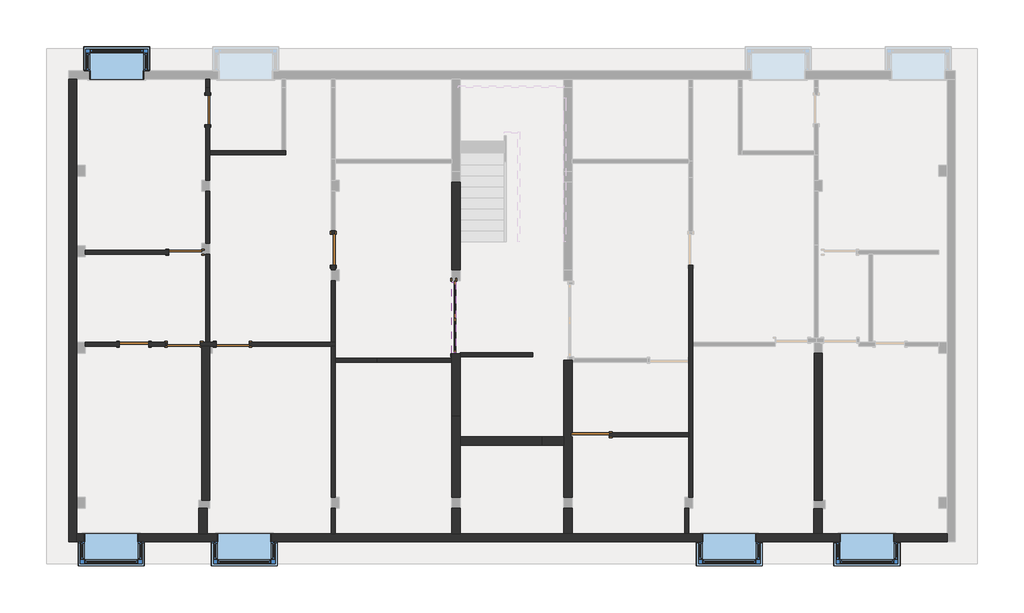
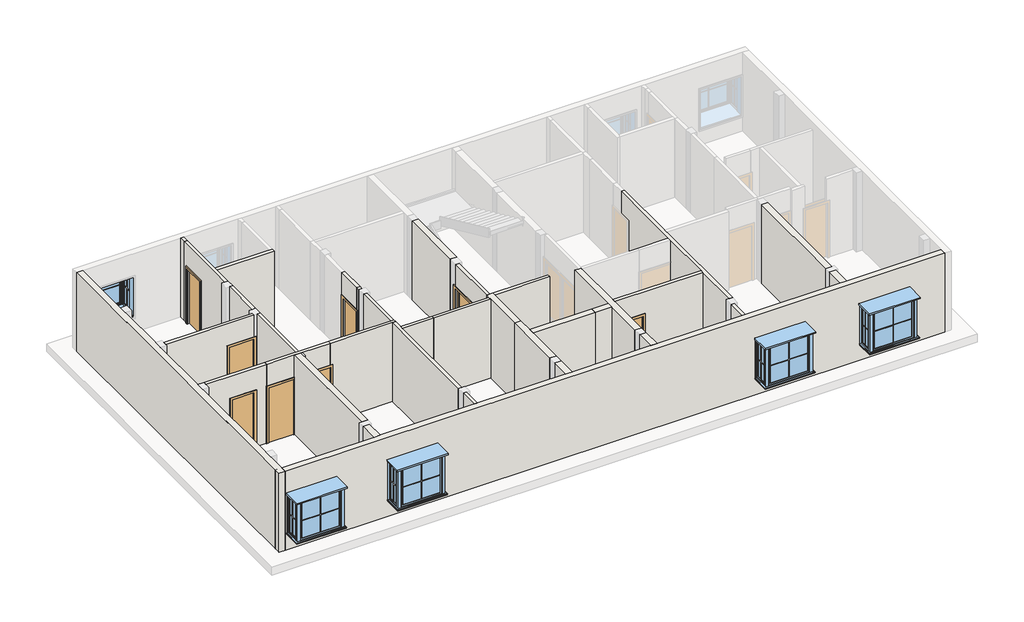
# One storey, part 1 of 3: 36 walls, 8 doors, 5 windows.
"""IFC4 building model written with IfcOpenShell, lengths in millimetres."""

from ifc_helpers import new_model, si_unit, frame, origin, place, context, project, spatial, polyline, outline, extrude, faceted_brep, transform, mapped, element, save
from components import door_b125cbd4, m_door_single_panel_05506f71, door_07b5d71c, door_4c0a2014, door_82def9da, m_door_single_panel_3_x7_f8176753, m_door_single_panel_3_x7_ebb67e73, window_19bbd869

model = new_model("IFC4")

# Units and contexts
model_context = context("Model", 3, world=origin())
ifc_project = project(units=[si_unit("LENGTHUNIT", "METRE", prefix="MILLI")], contexts=[model_context])

# Site, building, storey
site = spatial("IfcSite", under=ifc_project)
building = spatial("IfcBuilding", under=site)
storey = spatial("IfcBuildingStorey", under=building, Elevation=19202.4)

# Doors
placement = place(None, origin())
door_shape = door_b125cbd4(model_context)
element("IfcDoor", 1, ObjectType="M_Door-Double-Glass : 6'7\"X7'", at=placement, inside=storey, context=model_context, shape_type="MappedRepresentation", body=[
    mapped(door_shape, transform((-2022.6300498, 1267.5192699, 19202.4), x_axis=(0.0, 1.0, 0.0), y_axis=(-1.0, 0.0, 0.0), z_axis=(0.0, 0.0, 1.0))),
])
m_door_single_panel_shape = m_door_single_panel_05506f71(model_context)
element("IfcDoor", 2, ObjectType="M_Door-Single-Panel", at=placement, inside=storey, context=model_context, shape_type="MappedRepresentation", body=[
    mapped(m_door_single_panel_shape, transform((1745.3012085, -1975.7432663, 19202.4), x_axis=(-1.0, 0.0, 0.0), y_axis=(0.0, -1.0, 0.0), z_axis=(0.0, 0.0, 1.0))),
])
door_2_shape = door_07b5d71c(model_context)
element("IfcDoor", 3, ObjectType="M_Door-Single-Panel : 2'10\"X7' 2", at=placement, inside=storey, context=model_context, shape_type="MappedRepresentation", body=[
    mapped(door_2_shape, transform((-5360.3487995, 3142.9626891, 19202.4), x_axis=(0.0, -1.0, 0.0), y_axis=(1.0, 0.0, 0.0), z_axis=(0.0, 0.0, 1.0))),
])
door_3_shape = door_4c0a2014(model_context)
element("IfcDoor", 4, ObjectType="M_Door-Single-Panel : 2'8\"X7'", at=placement, inside=storey, context=model_context, shape_type="MappedRepresentation", body=[
    mapped(door_3_shape, transform((-10873.4462614, 526.1567334, 19202.4), x_axis=(1.0, 0.0, 0.0), y_axis=(0.0, 1.0, 0.0), z_axis=(0.0, 0.0, 1.0))),
])
door_4_shape = door_82def9da(model_context)
element("IfcDoor", 5, ObjectType="M_Door-Single-Panel : 2'8\"X7'", at=placement, inside=storey, context=model_context, shape_type="MappedRepresentation", body=[
    mapped(door_4_shape, transform((-8827.4487992, 7008.6751452, 19202.4), x_axis=(0.0, 1.0, 0.0), y_axis=(-1.0, 0.0, 0.0), z_axis=(0.0, 0.0, 1.0))),
])
m_door_single_panel_3_x7_shape = m_door_single_panel_3_x7_f8176753(model_context)
element("IfcDoor", 6, ObjectType="M_Door-Single-Panel : 3'X7'", at=placement, inside=storey, context=model_context, shape_type="MappedRepresentation", body=[
    mapped(m_door_single_panel_3_x7_shape, transform((-9456.0987989, 3078.8567332, 19202.4), x_axis=(1.0, 0.0, 0.0), y_axis=(0.0, 1.0, 0.0), z_axis=(0.0, 0.0, 1.0))),
])
element("IfcDoor", 7, ObjectType="M_Door-Single-Panel : 3'X7'", at=placement, inside=storey, context=model_context, shape_type="MappedRepresentation", body=[
    mapped(m_door_single_panel_3_x7_shape, transform((-8144.8381465, 526.1567334, 19202.4), x_axis=(-1.0, 0.0, 0.0), y_axis=(0.0, -1.0, 0.0), z_axis=(0.0, 0.0, 1.0))),
])
m_door_single_panel_3_x7_2_shape = m_door_single_panel_3_x7_ebb67e73(model_context)
element("IfcDoor", 8, ObjectType="M_Door-Single-Panel : 3'X7'", at=placement, inside=storey, context=model_context, shape_type="MappedRepresentation", body=[
    mapped(m_door_single_panel_3_x7_2_shape, transform((-9494.1987992, 526.1567334, 19202.4), x_axis=(1.0, 0.0, 0.0), y_axis=(0.0, 1.0, 0.0), z_axis=(0.0, 0.0, 1.0))),
])

# Walls
element("IfcWall", 9, ObjectType="4.5\"", at=placement, inside=storey, context=model_context, shape_type="SweptSolid", body=[
    extrude(outline(polyline([(2711.1626891, 22250.4), (3671.8272228, 22250.4), (3671.8272228, 19202.4), (3574.7626891, 19202.4), (3574.7626891, 21336.0), (2711.1626891, 21336.0), (2711.1626891, 22250.4)])), frame((-5417.4987995, 0.0, 0.0), z_axis=(1.0, 0.0, 0.0), x_axis=(0.0, 1.0, 0.0)), (0.0, 0.0, 1.0), 114.3),
])
element("IfcWall", 10, ObjectType="4.5\"", at=placement, inside=storey, context=model_context, shape_type="Brep", body=[
    faceted_brep([(-7690.1644155, 469.0067334, 22250.4), (-8713.148796, 469.0067334, 22250.4), (-8771.750543, 469.0067334, 22250.4), (-9000.350543, 469.0067334, 22250.4), (-10009.8462614, 469.0067334, 22250.4), (-10009.8462614, 469.0067334, 19202.4), (-9951.3987992, 469.0067334, 19202.4), (-9951.3987992, 469.0067334, 21336.0), (-9036.9987992, 469.0067334, 21336.0), (-9036.9987992, 469.0067334, 19202.4), (-9000.350543, 469.0067334, 19202.4), (-8771.750543, 469.0067334, 19202.4), (-8713.148796, 469.0067334, 19202.4), (-8602.0381465, 469.0067334, 19202.4), (-8602.0381465, 469.0067334, 21336.0), (-7690.1644155, 469.0067334, 21336.0), (-10009.8462614, 583.3067334, 22250.4), (-7690.1644155, 583.3067334, 22250.4), (-7690.1644155, 583.3067334, 21336.0), (-8602.0381465, 583.3067334, 21336.0), (-8602.0381465, 583.3067334, 19202.4), (-9036.9987992, 583.3067334, 19202.4), (-9036.9987992, 583.3067334, 21336.0), (-9951.3987992, 583.3067334, 21336.0), (-9951.3987992, 583.3067334, 19202.4), (-10009.8462614, 583.3067334, 19202.4)], [[[0, 1, 2, 3, 4, 5, 6, 7, 8, 9, 10, 11, 12, 13, 14, 15]], [[16, 17, 18, 19, 20, 21, 22, 23, 24, 25]], [[5, 25, 24, 6]], [[9, 21, 20, 13, 12, 11, 10]], [[17, 0, 15, 18]], [[4, 3, 2, 1, 0, 17, 16]], [[5, 4, 16, 25]], [[8, 22, 21, 9]], [[7, 23, 22, 8]], [[23, 7, 6, 24]], [[19, 14, 13, 20]], [[14, 19, 18, 15]]]),
])
element("IfcWall", 11, ObjectType="4.5\"", at=placement, inside=storey, context=model_context, shape_type="SweptSolid", body=[
    extrude(outline(polyline([(22250.4, 4475.8012082), (22250.4, 1250.0012085), (21336.0, 1250.0012085), (21336.0, 2278.7012085), (19202.4, 2278.7012085), (19202.4, 4475.8012082), (22250.4, 4475.8012082)])), frame((0.0, -2032.8932663, 0.0), z_axis=(0.0, 1.0, 0.0), x_axis=(0.0, 0.0, 1.0)), (0.0, 0.0, 1.0), 114.3),
])
element("IfcWall", 12, ObjectType="4.5\"", at=placement, inside=storey, context=model_context, shape_type="Brep", body=[
    faceted_brep([(-5417.4987995, 469.0067334, 19202.4), (-5417.4987995, -3709.2932193, 19202.4), (-5417.4987995, -3709.2932193, 22250.4), (-5417.4987995, 469.0067334, 22250.4), (-5303.1987995, 469.0067334, 19202.4), (-5303.1987995, 469.0067334, 22250.4), (-5303.1987995, 148.1078621, 22250.4), (-5303.1987995, 33.8078621, 22250.4), (-5303.1987995, -3709.2932193, 22250.4), (-5303.1987995, -3709.2932193, 19202.4), (-5303.1987995, 33.8078621, 19202.4), (-5303.1987995, 148.1078621, 19202.4)], [[[0, 1, 2, 3]], [[4, 5, 6, 7, 8, 9, 10, 11]], [[1, 0, 4, 11, 10, 9]], [[2, 1, 9, 8]], [[3, 2, 8, 7, 6, 5]], [[0, 3, 5, 4]]]),
])
element("IfcWall", 13, ObjectType="4.5\"", at=placement, inside=storey, context=model_context, shape_type="SweptSolid", body=[
    extrude(outline(polyline([(-5417.4987963, -4712.5932661), (-5417.4987963, -4014.0932193), (-5303.1987963, -4014.0932193), (-5303.1987963, -4712.5932661), (-5417.4987963, -4712.5932661)])), frame((0.0, 0.0, 19202.4), z_axis=(0.0, 0.0, 1.0), x_axis=(1.0, 0.0, 0.0)), (0.0, 0.0, 1.0), 3048.0),
])
element("IfcWall", 14, ObjectType="4.5\"", at=placement, inside=storey, context=model_context, shape_type="SweptSolid", body=[
    extrude(outline(polyline([(4361.5012082, -4712.5932661), (4361.5012082, -4014.0932193), (4475.8012082, -4014.0932193), (4475.8012082, -4712.5932661), (4361.5012082, -4712.5932661)])), frame((0.0, 0.0, 19202.4), z_axis=(0.0, 0.0, 1.0), x_axis=(1.0, 0.0, 0.0)), (0.0, 0.0, 1.0), 3048.0),
])
element("IfcWall", 15, ObjectType="4.5\"", at=placement, inside=storey, context=model_context, shape_type="SweptSolid", body=[
    extrude(outline(polyline([(-8770.2987992, 7860.4067329), (-8770.2987992, 7631.8067329), (-8884.5987992, 7631.8067329), (-8884.5987992, 7860.4067329), (-8770.2987992, 7860.4067329)])), frame((0.0, 0.0, 19202.4), z_axis=(0.0, 0.0, 1.0), x_axis=(1.0, 0.0, 0.0)), (0.0, 0.0, 1.0), 3048.0),
])
element("IfcWall", 16, ObjectType="4.5\"", at=placement, inside=storey, context=model_context, shape_type="SweptSolid", body=[
    extrude(outline(polyline([(-5303.1987995, 148.1078621), (-4161.4090098, 148.1078621), (-4161.4090098, 33.8078621), (-5303.1987995, 33.8078621), (-5303.1987995, 148.1078621)])), frame((0.0, 0.0, 19202.4), z_axis=(0.0, 0.0, 1.0), x_axis=(1.0, 0.0, 0.0)), (0.0, 0.0, 1.0), 3048.0),
])
element("IfcWall", 17, ObjectType="4.5\"", at=placement, inside=storey, context=model_context, shape_type="Brep", body=[
    faceted_brep([(154.7082462, 294.3817656, 19202.4), (-1848.7987998, 294.3817656, 19202.4), (-1848.7987998, 294.3817656, 21336.0), (-1848.7987998, 294.3817656, 22250.4), (154.7082462, 294.3817656, 22250.4), (154.7082462, 180.0817656, 19202.4), (154.7082462, 180.0817656, 22250.4), (-1848.7987998, 180.0817656, 22250.4), (-1848.7987998, 180.0817656, 19202.4), (-1848.7987998, 264.2192699, 19202.4)], [[[0, 1, 2, 3, 4]], [[5, 6, 7, 8]], [[1, 0, 5, 8, 9]], [[4, 3, 7, 6]], [[0, 4, 6, 5]], [[3, 2, 1, 9, 8, 7]]]),
])
element("IfcWall", 18, ObjectType="4.5\"", at=placement, inside=storey, context=model_context, shape_type="SweptSolid", body=[
    extrude(outline(polyline([(-1963.0987998, 2240.6567742), (-1963.0987998, 294.3817656), (-2077.3987998, 294.3817656), (-2077.3987998, 2240.6567742), (-1963.0987998, 2240.6567742)])), frame((0.0, 0.0, 21336.0), z_axis=(0.0, 0.0, 1.0), x_axis=(1.0, 0.0, 0.0)), (0.0, 0.0, 1.0), 914.4),
])
element("IfcWall", 19, ObjectType="4.5\" 2", at=placement, inside=storey, context=model_context, shape_type="SweptSolid", body=[
    extrude(outline(polyline([(22250.4, -8998.8987989), (22250.4, -12224.6987989), (19202.4, -12224.6987989), (19202.4, -9913.2987989), (21336.0, -9913.2987989), (21336.0, -8998.8987989), (22250.4, -8998.8987989)])), frame((0.0, 3021.7067332, 0.0), z_axis=(0.0, 1.0, 0.0), x_axis=(0.0, 0.0, 1.0)), (0.0, 0.0, 1.0), 114.3),
])
element("IfcWall", 20, ObjectType="4.5\" 2", at=placement, inside=storey, context=model_context, shape_type="SweptSolid", body=[
    extrude(outline(polyline([(-8770.2987992, 4761.606733), (-8770.2987992, 3326.5067332), (-8884.5987992, 3326.5067332), (-8884.5987992, 4761.606733), (-8770.2987992, 4761.606733)])), frame((0.0, 0.0, 19202.4), z_axis=(0.0, 0.0, 1.0), x_axis=(1.0, 0.0, 0.0)), (0.0, 0.0, 1.0), 3048.0),
])
element("IfcWall", 21, ObjectType="4.5\" 2", at=placement, inside=storey, context=model_context, shape_type="Brep", body=[
    faceted_brep([(-8770.2987992, 7415.0751452, 21336.0), (-8770.2987992, 7415.0751452, 19202.4), (-8770.2987992, 7631.8067329, 19202.4), (-8770.2987992, 7631.8067329, 22250.4), (-8770.2987992, 5879.2067329, 22250.4), (-8770.2987992, 5764.9067329, 22250.4), (-8770.2987992, 5066.406733, 22250.4), (-8770.2987992, 5066.406733, 19202.4), (-8770.2987992, 5764.9067329, 19202.4), (-8770.2987992, 5879.2067329, 19202.4), (-8770.2987992, 6602.2751452, 19202.4), (-8770.2987992, 6602.2751452, 21336.0), (-8884.5987992, 7631.8067329, 19202.4), (-8884.5987992, 7415.0751452, 19202.4), (-8884.5987992, 7415.0751452, 21336.0), (-8884.5987992, 6602.2751452, 21336.0), (-8884.5987992, 6602.2751452, 19202.4), (-8884.5987992, 5066.406733, 19202.4), (-8884.5987992, 5066.406733, 22250.4), (-8884.5987992, 7631.8067329, 22250.4)], [[[0, 1, 2, 3, 4, 5, 6, 7, 8, 9, 10, 11]], [[12, 13, 14, 15, 16, 17, 18, 19]], [[2, 1, 13, 12]], [[10, 9, 8, 7, 17, 16]], [[3, 2, 12, 19]], [[6, 5, 4, 3, 19, 18]], [[7, 6, 18, 17]], [[14, 13, 1, 0]], [[15, 14, 0, 11]], [[16, 15, 11, 10]]]),
])
element("IfcWall", 22, ObjectType="4.5\" 2", at=placement, inside=storey, context=model_context, shape_type="Brep", body=[
    faceted_brep([(-8770.2987992, 5764.9067329, 19202.4), (-6674.7987994, 5764.9067329, 19202.4), (-6674.7987994, 5764.9067329, 22250.4), (-8770.2987992, 5764.9067329, 22250.4), (-8770.2987992, 5879.2067329, 19202.4), (-8770.2987992, 5879.2067329, 22250.4), (-6789.0987994, 5879.2067329, 22250.4), (-6674.7987994, 5879.2067329, 22250.4), (-6674.7987994, 5879.2067329, 19202.4), (-6789.0987994, 5879.2067329, 19202.4)], [[[0, 1, 2, 3]], [[4, 5, 6, 7, 8, 9]], [[1, 0, 4, 9, 8]], [[3, 2, 7, 6, 5]], [[0, 3, 5, 4]], [[2, 1, 8, 7]]]),
])
element("IfcWall", 23, ObjectType="4.5\" 2", at=placement, inside=storey, context=model_context, shape_type="SweptSolid", body=[
    extrude(outline(polyline([(21336.0, -10467.0462614), (19202.4, -10467.0462614), (19202.4, -10009.8462614), (22250.4, -10009.8462614), (22250.4, -12224.6987989), (19202.4, -12224.6987989), (19202.4, -11279.8462614), (21336.0, -11279.8462614), (21336.0, -10467.0462614)])), frame((0.0, 469.0067334, 0.0), z_axis=(0.0, 1.0, 0.0), x_axis=(0.0, 0.0, 1.0)), (0.0, 0.0, 1.0), 114.3),
])
element("IfcWall", 24, ObjectType="4.5\" 2", at=placement, inside=storey, context=model_context, shape_type="SweptSolid", body=[
    extrude(outline(polyline([(-8770.298796, 3021.7067332), (-8770.298796, 583.3067804), (-8884.598796, 583.3067804), (-8884.598796, 3021.7067332), (-8770.298796, 3021.7067332)])), frame((0.0, 0.0, 19202.4), z_axis=(0.0, 0.0, 1.0), x_axis=(1.0, 0.0, 0.0)), (0.0, 0.0, 1.0), 3048.0),
])
element("IfcWall", 25, ObjectType="4.5\" 2", at=placement, inside=storey, context=model_context, shape_type="Brep", body=[
    faceted_brep([(-5303.1987995, 469.0067334, 22250.4), (-5417.4987995, 469.0067334, 22250.4), (-7690.1644155, 469.0067334, 22250.4), (-7690.1644155, 469.0067334, 21336.0), (-7687.6381465, 469.0067334, 21336.0), (-7687.6381465, 469.0067334, 19202.4), (-5417.4987995, 469.0067334, 19202.4), (-5303.1987995, 469.0067334, 19202.4), (-7690.1644155, 583.3067334, 22250.4), (-5417.4987995, 583.3067334, 22250.4), (-5303.1987995, 583.3067334, 22250.4), (-5303.1987995, 583.3067334, 19202.4), (-5417.4987995, 583.3067334, 19202.4), (-7687.6381465, 583.3067334, 19202.4), (-7687.6381465, 583.3067334, 21336.0), (-7690.1644155, 583.3067334, 21336.0)], [[[0, 1, 2, 3, 4, 5, 6, 7]], [[8, 9, 10, 11, 12, 13, 14, 15]], [[11, 7, 6, 5, 13, 12]], [[2, 1, 0, 10, 9, 8]], [[2, 8, 15, 3]], [[0, 7, 11, 10]], [[14, 4, 3, 15]], [[4, 14, 13, 5]]]),
])
element("IfcWall", 26, ObjectType="4.5\" 2", at=placement, inside=storey, context=model_context, shape_type="SweptSolid", body=[
    extrude(outline(polyline([(-5303.1987995, 2285.1067802), (-5303.1987995, 583.3067334), (-5417.4987995, 583.3067334), (-5417.4987995, 2285.1067802), (-5303.1987995, 2285.1067802)])), frame((0.0, 0.0, 19202.4), z_axis=(0.0, 0.0, 1.0), x_axis=(1.0, 0.0, 0.0)), (0.0, 0.0, 1.0), 3048.0),
])
element("IfcWall", 27, ObjectType="4.5\" 2", at=placement, inside=storey, context=model_context, shape_type="Brep", body=[
    faceted_brep([(-5303.1987995, 2589.9067802, 19202.4), (-5303.1987995, 2711.1626891, 19202.4), (-5303.1987995, 2711.1626891, 21336.0), (-5303.1987995, 2711.1626891, 22250.4), (-5303.1987995, 2589.9067802, 22250.4), (-5417.4987995, 2589.9067802, 19202.4), (-5417.4987995, 2589.9067802, 22250.4), (-5417.4987995, 2711.1626891, 22250.4), (-5417.4987995, 2711.1626891, 21336.0), (-5417.4987995, 2711.1626891, 19202.4)], [[[0, 1, 2, 3, 4]], [[5, 6, 7, 8, 9]], [[1, 0, 5, 9]], [[3, 2, 1, 9, 8, 7]], [[4, 3, 7, 6]], [[0, 4, 6, 5]]]),
])
element("IfcWall", 28, ObjectType="4.5\" 2", at=placement, inside=storey, context=model_context, shape_type="Brep", body=[
    faceted_brep([(4475.8012082, -3709.2932193, 19202.4), (4475.8012082, -3709.2932193, 22250.4), (4475.8012082, -2032.8932663, 22250.4), (4475.8012082, -1918.5932663, 22250.4), (4475.8012082, 33.8078621, 22250.4), (4475.8012082, 148.1078621, 22250.4), (4475.8012082, 3132.0737955, 22250.4), (4475.8012082, 3132.0737955, 21336.0), (4475.8012082, 2711.1626891, 21336.0), (4475.8012082, 2711.1626891, 19202.4), (4475.8012082, 148.1078621, 19202.4), (4475.8012082, 33.8078621, 19202.4), (4475.8012082, -1918.5932663, 19202.4), (4475.8012082, -2032.8932663, 19202.4), (4590.1012082, -3709.2932193, 22250.4), (4590.1012082, -3709.2932193, 19202.4), (4590.1012082, 469.0067334, 19202.4), (4590.1012082, 583.3067334, 19202.4), (4590.1012082, 2711.1626891, 19202.4), (4590.1012082, 2711.1626891, 21336.0), (4590.1012082, 3132.0737955, 21336.0), (4590.1012082, 3132.0737955, 22250.4), (4590.1012082, 583.3067334, 22250.4), (4590.1012082, 469.0067334, 22250.4)], [[[0, 1, 2, 3, 4, 5, 6, 7, 8, 9, 10, 11, 12, 13]], [[14, 15, 16, 17, 18, 19, 20, 21, 22, 23]], [[15, 0, 13, 12, 11, 10, 9, 18, 17, 16]], [[1, 0, 15, 14]], [[6, 5, 4, 3, 2, 1, 14, 23, 22, 21]], [[6, 21, 20, 7]], [[8, 19, 18, 9]], [[19, 8, 7, 20]]]),
])
element("IfcWall", 29, ObjectType="4.5\" 2", at=placement, inside=storey, context=model_context, shape_type="SweptSolid", body=[
    extrude(outline(polyline([(-2077.3987998, 33.8078621), (-4161.4090098, 33.8078621), (-4161.4090098, 148.1078621), (-2077.3987998, 148.1078621), (-2077.3987998, 33.8078621)])), frame((0.0, 0.0, 19202.4), z_axis=(0.0, 0.0, 1.0), x_axis=(1.0, 0.0, 0.0)), (0.0, 0.0, 1.0), 3048.0),
])
element("IfcWall", 30, ObjectType="9\"", at=placement, inside=storey, context=model_context, shape_type="Brep", body=[
    faceted_brep([(-12453.2987957, -4941.1932661, 19202.4), (-12453.2987957, -4712.5932661, 19202.4), (-12453.2987957, -4014.0932671, 19202.4), (-12453.2987957, -3709.2932671, 19202.4), (-12453.2987957, 278.5067334, 19202.4), (-12453.2987957, 583.3067334, 19202.4), (-12453.2987957, 2951.8567332, 19202.4), (-12453.2987957, 3256.6567332, 19202.4), (-12453.2987957, 5174.3567339, 19202.4), (-12453.2987957, 5479.1567339, 19202.4), (-12453.2987957, 7860.4067329, 19202.4), (-12453.2987957, 7860.4067329, 22250.4), (-12453.2987957, 5479.1567339, 22250.4), (-12453.2987957, 5174.3567339, 22250.4), (-12453.2987957, 3256.6567332, 22250.4), (-12453.2987957, 2951.8567332, 22250.4), (-12453.2987957, 583.3067334, 22250.4), (-12453.2987957, 278.5067334, 22250.4), (-12453.2987957, -3709.2932671, 22250.4), (-12453.2987957, -4014.0932671, 22250.4), (-12453.2987957, -4712.5932661, 22250.4), (-12453.2987957, -4941.1932661, 22250.4), (-12681.8987957, -4941.1932661, 19202.4), (-12681.8987957, -4941.1932661, 22250.4), (-12681.8987957, 7860.4067329, 22250.4), (-12681.8987957, 7860.4067329, 19202.4)], [[[0, 1, 2, 3, 4, 5, 6, 7, 8, 9, 10, 11, 12, 13, 14, 15, 16, 17, 18, 19, 20, 21]], [[22, 23, 24, 25]], [[10, 9, 8, 7, 6, 5, 4, 3, 2, 1, 0, 22, 25]], [[21, 20, 19, 18, 17, 16, 15, 14, 13, 12, 11, 24, 23]], [[11, 10, 25, 24]], [[0, 21, 23, 22]]]),
])
element("IfcWall", 31, ObjectType="9\"", at=placement, inside=storey, context=model_context, shape_type="Brep", body=[
    faceted_brep([(-12453.2987957, -4712.5932661, 19202.4), (-12453.2987957, -4014.0932671, 19202.4), (-12453.2987957, -3709.2932671, 19202.4), (-12453.2987957, 278.5067334, 19202.4), (-12453.2987957, 583.3067334, 19202.4), (-12453.2987957, 2951.8567332, 19202.4), (-12453.2987957, 3256.6567332, 19202.4), (-12453.2987957, 5174.3567339, 19202.4), (-12453.2987957, 5479.1567339, 19202.4), (-12453.2987957, 7860.4067329, 19202.4), (-12453.2987957, 7860.4067329, 22250.4), (-12453.2987957, 5479.1567339, 22250.4), (-12453.2987957, 5174.3567339, 22250.4), (-12453.2987957, 3256.6567332, 22250.4), (-12453.2987957, 2951.8567332, 22250.4), (-12453.2987957, 583.3067334, 22250.4), (-12453.2987957, 278.5067334, 22250.4), (-12453.2987957, -3709.2932671, 22250.4), (-12453.2987957, -4014.0932671, 22250.4), (-12453.2987957, -4712.5932661, 22250.4), (-12681.8987957, -4712.5932661, 19202.4), (-12681.8987957, -4712.5932661, 22250.4), (-12681.8987957, 7860.4067329, 22250.4), (-12681.8987957, 7860.4067329, 19202.4)], [[[0, 1, 2, 3, 4, 5, 6, 7, 8, 9, 10, 11, 12, 13, 14, 15, 16, 17, 18, 19]], [[20, 21, 22, 23]], [[9, 8, 7, 6, 5, 4, 3, 2, 1, 0, 20, 23]], [[19, 18, 17, 16, 15, 14, 13, 12, 11, 10, 22, 21]], [[10, 9, 23, 22]], [[0, 19, 21, 20]]]),
])
element("IfcWall", 32, ObjectType="9\"", at=placement, inside=storey, context=model_context, shape_type="Brep", body=[
    faceted_brep([(-9000.350543, 469.0067334, 19202.4), (-9000.350543, -3785.4932196, 19202.4), (-9000.350543, -3785.4932196, 22250.4), (-9000.350543, 469.0067334, 22250.4), (-8771.750543, 469.0067334, 19202.4), (-8771.750543, 469.0067334, 22250.4), (-8771.750543, 278.5067334, 22250.4), (-8771.750543, -3785.4932196, 22250.4), (-8771.750543, -3785.4932196, 19202.4), (-8771.750543, 278.5067334, 19202.4)], [[[0, 1, 2, 3]], [[4, 5, 6, 7, 8, 9]], [[1, 0, 4, 9, 8]], [[2, 1, 8, 7]], [[3, 2, 7, 6, 5]], [[0, 3, 5, 4]]]),
])
element("IfcWall", 33, ObjectType="9\"", at=placement, inside=storey, context=model_context, shape_type="Brep", body=[
    faceted_brep([(-2077.3987998, -1469.0258023, 19202.4), (-2077.3987998, -1469.0258023, 22250.4), (-2077.3987998, 33.8078621, 22250.4), (-2077.3987998, 148.1078621, 22250.4), (-2077.3987998, 294.3817656, 22250.4), (-2077.3987998, 294.3817656, 21336.0), (-2077.3987998, 264.2192699, 21336.0), (-2077.3987998, 264.2192699, 19202.4), (-2077.3987998, 148.1078621, 19202.4), (-2077.3987998, 33.8078621, 19202.4), (-1848.7987998, -1469.0258023, 22250.4), (-1848.7987998, -1469.0258023, 19202.4), (-1848.7987998, 180.0817656, 19202.4), (-1848.7987998, 264.2192699, 19202.4), (-1848.7987998, 264.2192699, 21336.0), (-1848.7987998, 294.3817656, 21336.0), (-1848.7987998, 294.3817656, 22250.4), (-1848.7987998, 180.0817656, 22250.4), (-1963.0987998, 294.3817656, 22250.4), (-1963.0987998, 294.3817656, 21336.0)], [[[0, 1, 2, 3, 4, 5, 6, 7, 8, 9]], [[10, 11, 12, 13, 14, 15, 16, 17]], [[11, 0, 9, 8, 7, 13, 12]], [[1, 0, 11, 10]], [[4, 3, 2, 1, 10, 17, 16, 18]], [[4, 18, 16, 15, 19, 5]], [[14, 6, 5, 19, 15]], [[6, 14, 13, 7]]]),
])
element("IfcWall", 34, ObjectType="9\"", at=placement, inside=storey, context=model_context, shape_type="Brep", body=[
    faceted_brep([(-2077.3987998, -1469.0258023, 19202.4), (-2077.3987998, -3709.2932663, 19202.4), (-2077.3987998, -3709.2932663, 22250.4), (-2077.3987998, -1469.0258023, 22250.4), (-1848.7987998, -1469.0258023, 19202.4), (-1848.7987998, -1469.0258023, 22250.4), (-1848.7987998, -2032.8932663, 22250.4), (-1848.7987998, -2261.4932663, 22250.4), (-1848.7987998, -3709.2932663, 22250.4), (-1848.7987998, -3709.2932663, 19202.4), (-1848.7987998, -2261.4932663, 19202.4), (-1848.7987998, -2032.8932663, 19202.4)], [[[0, 1, 2, 3]], [[4, 5, 6, 7, 8, 9, 10, 11]], [[1, 0, 4, 11, 10, 9]], [[2, 1, 9, 8]], [[3, 2, 8, 7, 6, 5]], [[0, 3, 5, 4]]]),
])
element("IfcWall", 35, ObjectType="9\"", at=placement, inside=storey, context=model_context, shape_type="SweptSolid", body=[
    extrude(outline(polyline([(1021.4012085, -2261.4932663), (412.152227, -2261.4932663), (412.152227, -2032.8932663), (1021.4012085, -2032.8932663), (1021.4012085, -2261.4932663)])), frame((0.0, 0.0, 19202.4), z_axis=(0.0, 0.0, 1.0), x_axis=(1.0, 0.0, 0.0)), (0.0, 0.0, 1.0), 3048.0),
])
element("IfcWall", 36, ObjectType="9\"", at=placement, inside=storey, context=model_context, shape_type="Brep", body=[
    faceted_brep([(1021.4012085, 90.9578621, 19202.4), (1021.4012085, -2032.8932663, 19202.4), (1021.4012085, -2261.4932663, 19202.4), (1021.4012085, -3709.2932193, 19202.4), (1021.4012085, -3709.2932193, 22250.4), (1021.4012085, -2261.4932663, 22250.4), (1021.4012085, -2032.8932663, 22250.4), (1021.4012085, 90.9578621, 22250.4), (1250.0012085, -3709.2932193, 22250.4), (1250.0012085, -3709.2932193, 19202.4), (1250.0012085, -2032.8932663, 19202.4), (1250.0012085, -2032.8932663, 21336.0), (1250.0012085, -1918.5932663, 21336.0), (1250.0012085, -1918.5932663, 19202.4), (1250.0012085, 33.8078621, 19202.4), (1250.0012085, 90.9578621, 19202.4), (1250.0012085, 90.9578621, 22250.4), (1250.0012085, 33.8078621, 22250.4), (1250.0012085, -1918.5932663, 22250.4), (1250.0012085, -2032.8932663, 22250.4), (1158.0082462, 90.9578621, 19202.4), (1211.9012085, -1918.5932663, 19202.4), (1211.9012085, -2032.8932663, 19202.4), (1158.0082462, 90.9578621, 22250.4), (1211.9012085, -1918.5932663, 21336.0), (1211.9012085, -2032.8932663, 21336.0)], [[[0, 1, 2, 3, 4, 5, 6, 7]], [[8, 9, 10, 11, 12, 13, 14, 15, 16, 17, 18, 19]], [[3, 2, 1, 0, 20, 15, 14, 13, 21, 22, 10, 9]], [[4, 3, 9, 8]], [[7, 6, 5, 4, 8, 19, 18, 17, 16, 23]], [[0, 7, 23, 16, 15, 20]], [[24, 21, 13, 12]], [[22, 25, 11, 10]], [[21, 24, 25, 22]], [[25, 24, 12, 11]]]),
])
element("IfcWall", 37, ObjectType="9\"", at=placement, inside=storey, context=model_context, shape_type="SweptSolid", body=[
    extrude(outline(polyline([(-2074.1417538, 2589.906774), (-2074.1417538, 5015.606774), (-1845.5417538, 5015.606774), (-1845.5417538, 2589.906774), (-2074.1417538, 2589.906774)])), frame((0.0, 0.0, 19202.4), z_axis=(0.0, 0.0, 1.0), x_axis=(1.0, 0.0, 0.0)), (0.0, 0.0, 1.0), 3048.0),
])
element("IfcWall", 38, ObjectType="9\"", at=placement, inside=storey, context=model_context, shape_type="SweptSolid", body=[
    extrude(outline(polyline([(7942.9012047, -3785.4932666), (7942.9012047, 278.5067334), (8171.5012047, 278.5067334), (8171.5012047, -3785.4932666), (7942.9012047, -3785.4932666)])), frame((0.0, 0.0, 19202.4), z_axis=(0.0, 0.0, 1.0), x_axis=(1.0, 0.0, 0.0)), (0.0, 0.0, 1.0), 3048.0),
])
element("IfcWall", 39, ObjectType="9\"", at=placement, inside=storey, context=model_context, shape_type="SweptSolid", body=[
    extrude(outline(polyline([(1021.4012085, -4712.5932661), (1021.4012085, -4014.0932193), (1250.0012085, -4014.0932193), (1250.0012085, -4712.5932661), (1021.4012085, -4712.5932661)])), frame((0.0, 0.0, 19202.4), z_axis=(0.0, 0.0, 1.0), x_axis=(1.0, 0.0, 0.0)), (0.0, 0.0, 1.0), 3048.0),
])
element("IfcWall", 40, ObjectType="9\"", at=placement, inside=storey, context=model_context, shape_type="SweptSolid", body=[
    extrude(outline(polyline([(7941.7646942, -4712.5932661), (7941.7646942, -4015.9914801), (8170.3646942, -4015.9914801), (8170.3646942, -4712.5932661), (7941.7646942, -4712.5932661)])), frame((0.0, 0.0, 19202.4), z_axis=(0.0, 0.0, 1.0), x_axis=(1.0, 0.0, 0.0)), (0.0, 0.0, 1.0), 3048.0),
])
element("IfcWall", 41, ObjectType="9\"", at=placement, inside=storey, context=model_context, shape_type="SweptSolid", body=[
    extrude(outline(polyline([(-2077.3987998, -4712.5932661), (-2077.3987998, -4014.0932663), (-1848.7987998, -4014.0932663), (-1848.7987998, -4712.5932661), (-2077.3987998, -4712.5932661)])), frame((0.0, 0.0, 19202.4), z_axis=(0.0, 0.0, 1.0), x_axis=(1.0, 0.0, 0.0)), (0.0, 0.0, 1.0), 3048.0),
])
element("IfcWall", 42, ObjectType="9\"", at=placement, inside=storey, context=model_context, shape_type="SweptSolid", body=[
    extrude(outline(polyline([(-9076.550543, -4712.5932661), (-9076.550543, -4014.0932196), (-8847.950543, -4014.0932196), (-8847.950543, -4712.5932661), (-9076.550543, -4712.5932661)])), frame((0.0, 0.0, 19202.4), z_axis=(0.0, 0.0, 1.0), x_axis=(1.0, 0.0, 0.0)), (0.0, 0.0, 1.0), 3048.0),
])
element("IfcWall", 43, ObjectType="9\"", at=placement, inside=storey, context=model_context, shape_type="SweptSolid", body=[
    extrude(outline(polyline([(-1848.7987998, -2032.8932663), (412.152227, -2032.8932663), (412.152227, -2261.4932663), (-1848.7987998, -2261.4932663), (-1848.7987998, -2032.8932663)])), frame((0.0, 0.0, 19202.4), z_axis=(0.0, 0.0, 1.0), x_axis=(1.0, 0.0, 0.0)), (0.0, 0.0, 1.0), 3048.0),
])
element("IfcWall", 44, ObjectType="9\" 2", at=placement, inside=storey, context=model_context, shape_type="Brep", body=[
    faceted_brep([(-12453.2987957, -4941.1932661, 19202.4), (11625.9012075, -4941.1932662, 19202.4), (11625.9012075, -4941.1932662, 22250.4), (-12453.2987957, -4941.1932661, 22250.4), (8658.6146942, -4941.1932661, 21353.2), (10158.6146942, -4941.1932661, 21353.2), (10158.6146942, -4941.1932661, 19802.4), (8658.6146942, -4941.1932661, 19802.4), (4849.7512082, -4941.1932661, 21353.2), (6349.7512082, -4941.1932661, 21353.2), (6349.7512082, -4941.1932661, 19802.4), (4849.7512082, -4941.1932661, 19802.4), (-8569.250543, -4941.1932661, 21353.2), (-7069.250543, -4941.1932661, 21353.2), (-7069.250543, -4941.1932661, 19802.4), (-8569.250543, -4941.1932661, 19802.4), (-12250.7987957, -4941.1932661, 21353.2), (-10750.7987957, -4941.1932661, 21353.2), (-10750.7987957, -4941.1932661, 19802.4), (-12250.7987957, -4941.1932661, 19802.4), (-12453.2987957, -4712.5932661, 19202.4), (-12453.2987957, -4712.5932661, 22250.4), (-9076.550543, -4712.5932661, 22250.4), (-8847.950543, -4712.5932661, 22250.4), (-5417.4987963, -4712.5932661, 22250.4), (-5303.1987963, -4712.5932661, 22250.4), (-2077.3987998, -4712.5932661, 22250.4), (-1848.7987998, -4712.5932661, 22250.4), (1021.4012085, -4712.5932661, 22250.4), (1250.0012085, -4712.5932661, 22250.4), (4361.5012082, -4712.5932661, 22250.4), (4475.8012082, -4712.5932661, 22250.4), (7941.7646942, -4712.5932661, 22250.4), (8170.3646942, -4712.5932661, 22250.4), (11625.9012075, -4712.5932662, 22250.4), (11625.9012075, -4712.5932662, 19202.4), (8170.3646942, -4712.5932661, 19202.4), (7941.7646942, -4712.5932661, 19202.4), (4475.8012082, -4712.5932661, 19202.4), (4361.5012082, -4712.5932661, 19202.4), (1250.0012085, -4712.5932661, 19202.4), (1021.4012085, -4712.5932661, 19202.4), (-1848.7987998, -4712.5932661, 19202.4), (-2077.3987998, -4712.5932661, 19202.4), (-5303.1987963, -4712.5932661, 19202.4), (-5417.4987963, -4712.5932661, 19202.4), (-8847.950543, -4712.5932661, 19202.4), (-9076.550543, -4712.5932661, 19202.4), (8658.6146942, -4712.5932661, 21353.2), (8658.6146942, -4712.5932661, 19802.4), (10158.6146942, -4712.5932661, 19802.4), (10158.6146942, -4712.5932661, 21353.2), (4849.7512082, -4712.5932661, 21353.2), (4849.7512082, -4712.5932661, 19802.4), (6349.7512082, -4712.5932661, 19802.4), (6349.7512082, -4712.5932661, 21353.2), (-8569.250543, -4712.5932661, 21353.2), (-8569.250543, -4712.5932661, 19802.4), (-7069.250543, -4712.5932661, 19802.4), (-7069.250543, -4712.5932661, 21353.2), (-12250.7987957, -4712.5932661, 21353.2), (-12250.7987957, -4712.5932661, 19802.4), (-10750.7987957, -4712.5932661, 19802.4), (-10750.7987957, -4712.5932661, 21353.2)], [[[0, 1, 2, 3], [4, 5, 6, 7], [8, 9, 10, 11], [12, 13, 14, 15], [16, 17, 18, 19]], [[20, 21, 22, 23, 24, 25, 26, 27, 28, 29, 30, 31, 32, 33, 34, 35, 36, 37, 38, 39, 40, 41, 42, 43, 44, 45, 46, 47], [48, 49, 50, 51], [52, 53, 54, 55], [56, 57, 58, 59], [60, 61, 62, 63]], [[1, 0, 20, 47, 46, 45, 44, 43, 42, 41, 40, 39, 38, 37, 36, 35]], [[3, 2, 34, 33, 32, 31, 30, 29, 28, 27, 26, 25, 24, 23, 22, 21]], [[2, 1, 35, 34]], [[0, 3, 21, 20]], [[49, 48, 4, 7]], [[50, 49, 7, 6]], [[51, 50, 6, 5]], [[48, 51, 5, 4]], [[53, 52, 8, 11]], [[54, 53, 11, 10]], [[55, 54, 10, 9]], [[52, 55, 9, 8]], [[57, 56, 12, 15]], [[58, 57, 15, 14]], [[59, 58, 14, 13]], [[56, 59, 13, 12]], [[61, 60, 16, 19]], [[62, 61, 19, 18]], [[63, 62, 18, 17]], [[60, 63, 17, 16]]]),
])

# Windows
window_shape = window_19bbd869(model_context)
element("IfcWindow", 45, ObjectType="4'.8\"x3'.8\"", at=placement, inside=storey, context=model_context, shape_type="MappedRepresentation", body=[
    mapped(window_shape, transform((-11500.7987957, -4826.8932661, 19202.4), x_axis=(-1.0, 0.0, 0.0), y_axis=(0.0, -1.0, 0.0), z_axis=(0.0, 0.0, 1.0))),
])
element("IfcWindow", 46, ObjectType="4'.8\"x3'.8\"", at=placement, inside=storey, context=model_context, shape_type="MappedRepresentation", body=[
    mapped(window_shape, transform((-7819.250543, -4826.8932661, 19202.4), x_axis=(-1.0, 0.0, 0.0), y_axis=(0.0, -1.0, 0.0), z_axis=(0.0, 0.0, 1.0))),
])
element("IfcWindow", 47, ObjectType="4'.8\"x3'.8\"", at=placement, inside=storey, context=model_context, shape_type="MappedRepresentation", body=[
    mapped(window_shape, transform((5599.7512082, -4826.8932661, 19202.4), x_axis=(-1.0, 0.0, 0.0), y_axis=(0.0, -1.0, 0.0), z_axis=(0.0, 0.0, 1.0))),
])
element("IfcWindow", 48, ObjectType="4'.8\"x3'.8\"", at=placement, inside=storey, context=model_context, shape_type="MappedRepresentation", body=[
    mapped(window_shape, transform((9408.6146942, -4826.8932661, 19202.4), x_axis=(-1.0, 0.0, 0.0), y_axis=(0.0, -1.0, 0.0), z_axis=(0.0, 0.0, 1.0))),
])
element("IfcWindow", 49, ObjectType="4'.8\"x3'.8\"", at=placement, inside=storey, context=model_context, shape_type="MappedRepresentation", body=[
    mapped(window_shape, transform((-11348.3987957, 7974.7067329, 19202.4), x_axis=(1.0, 0.0, 0.0), y_axis=(0.0, 1.0, 0.0), z_axis=(0.0, 0.0, 1.0))),
])

save(model, "model.ifc")

# Revit data of these elements
# Type "M_Door-Double-Glass : 6'7\"X7'"
#   Type Mark = "16"
#   Construction Type Id = "opn-d45"
#   Assembly Code = "C1020"
#   Analytic Construction = "Wood frame, double glass door "
#   W = 3' - 3 1/2"
#   Thickness = 0' - 1.9685"
#   Thermal Resistance (R) = 1.8150 (h·ft²·°F)/BTU
#   Swing Angle [instance default] = 90.00°
#   Heat Transfer Coefficient (U) = 0.5510 BTU/(h·ft²·°F)
#   Height = 7' - 0"
#   Bottom Rail = 0' - 3.93701"
#   Top Rail = 0' - 3.93701"
#   Stiles = 0' - 3.93701"
#   Trim Projection = 0' - 0.98425"
#   Trim Width = 0' - 3.14961"
#   Width = 6' - 7"
#   Define Thermal Properties by = 1
#   Glazing = Glass
#   Panel Material = Wood - Birch - Solid Stained Light Low Gloss
#   Trim Material = Paint - Sienna
#   Visual Light Transmittance = 0
#   Solar Heat Gain Coefficient = 0
#   Function = (empty or 0)
#   Wall Closure = (empty or 0)
# Type "M_Door-Single-Panel"
#   Type Mark = "14"
#   Construction Type Id = "DOOR"
#   Assembly Code = "C1020300"
#   Analytic Construction = "Wooden"
#   Thickness = 0' - 1.9685"
#   Thermal Resistance (R) = 2.5876 (h·ft²·°F)/BTU
#   Swing Angle [instance default] = 90.00°
#   Heat Transfer Coefficient (U) = 0.3865 BTU/(h·ft²·°F)
#   Height = 7' - 0"
#   Trim Projection Ext = 0' - 0.98425"
#   Trim Projection Int = 0' - 0.98425"
#   Trim Width = 0' - 3.14961"
#   Width = 3' - 6"
#   Define Thermal Properties by = 1
#   Panel Material = Wood - Birch - Solid Stained Light Low Gloss
#   Trim Material = Paint - Sienna
#   Visual Light Transmittance = 0
#   Solar Heat Gain Coefficient = 0
#   Function = (empty or 0)
#   Wall Closure = (empty or 0)
# Type "M_Door-Single-Panel : 2'10\"X7' 2"
#   Type Mark = "10"
#   Construction Type Id = "DOOR"
#   Assembly Code = "C1020300"
#   Analytic Construction = "Wooden"
#   Thickness = 0' - 1.9685"
#   Thermal Resistance (R) = 2.5876 (h·ft²·°F)/BTU
#   Swing Angle [instance default] = 90.00°
#   Heat Transfer Coefficient (U) = 0.3865 BTU/(h·ft²·°F)
#   Height = 7' - 0"
#   Trim Projection Ext = 0' - 0.98425"
#   Trim Projection Int = 0' - 0.98425"
#   Trim Width = 0' - 3.14961"
#   Width = 2' - 10"
#   Define Thermal Properties by = 1
#   Panel Material = Wood - Birch - Solid Stained Light Low Gloss
#   Trim Material = Paint - Sienna
#   Visual Light Transmittance = 0
#   Solar Heat Gain Coefficient = 0
#   Function = (empty or 0)
#   Wall Closure = (empty or 0)
# Type "M_Door-Single-Panel : 2'8\"X7'"
#   Type Mark = "9"
#   Construction Type Id = "DOOR"
#   Assembly Code = "C1020300"
#   Analytic Construction = "Wooden"
#   Thickness = 0' - 1.9685"
#   Thermal Resistance (R) = 2.5876 (h·ft²·°F)/BTU
#   Swing Angle [instance default] = 90.00°
#   Heat Transfer Coefficient (U) = 0.3865 BTU/(h·ft²·°F)
#   Height = 7' - 0"
#   Trim Projection Ext = 0' - 0.98425"
#   Trim Projection Int = 0' - 0.98425"
#   Trim Width = 0' - 3.14961"
#   Width = 2' - 8"
#   Define Thermal Properties by = 1
#   Panel Material = Wood - Birch - Solid Stained Light Low Gloss
#   Trim Material = Paint - Sienna
#   Visual Light Transmittance = 0
#   Solar Heat Gain Coefficient = 0
#   Function = (empty or 0)
#   Wall Closure = (empty or 0)
# Type "M_Door-Single-Panel : 3'X7'"
#   Type Mark = "11"
#   Construction Type Id = "DOOR"
#   Assembly Code = "C1020300"
#   Analytic Construction = "Wooden"
#   Thickness = 0' - 1.9685"
#   Thermal Resistance (R) = 2.5876 (h·ft²·°F)/BTU
#   Swing Angle [instance default] = 90.00°
#   Heat Transfer Coefficient (U) = 0.3865 BTU/(h·ft²·°F)
#   Height = 7' - 0"
#   Trim Projection Ext = 0' - 0.98425"
#   Trim Projection Int = 0' - 0.98425"
#   Trim Width = 0' - 3.14961"
#   Width = 3' - 0"
#   Define Thermal Properties by = 1
#   Panel Material = Wood - Birch - Solid Stained Light Low Gloss
#   Trim Material = Paint - Sienna
#   Visual Light Transmittance = 0
#   Solar Heat Gain Coefficient = 0
#   Function = (empty or 0)
#   Wall Closure = (empty or 0)
# Type "4.5\""
#   Assembly Code = "B2010"
#   Layers, outside or top first: 0' - 4 1/2" no material (function 1)
# Type "4.5\" 2"
#   Assembly Code = "B2010"
#   Layers, outside or top first: 0' - 4 1/2" no material (function 1)
# Type "9\""
#   Assembly Code = "B2010"
#   Layers, outside or top first: 0' - 9" no material (function 1)
# Type "9\" 2"
#   Assembly Code = "B2010"
#   Layers, outside or top first: 0' - 9" no material (function 1)
# Type "4'.8\"x3'.8\""
#   Type Mark = "20"
#   Fire Rating = "0.5h"
#   Assembly Code = "B2020100"
#   Analytic Construction = "1/8 in Pilkington single glazing"
#   Width = 4' - 11.05512"
#   Wall Thickness [instance default] = 0' - 5.90551"
#   Visual Light Transmittance = 0.9
#   Trim Width = 5' - 7.05512"
#   Trim Height = 4' - 11.05512"
#   Thermal Resistance (R) = 1.5394 (h·ft²·°F)/BTU
#   Solar Heat Gain Coefficient = 0.86
#   Rough Width = 4' - 11.64567"
#   Rough Height = 4' - 11.64567"
#   Height 1 = 5' - 1.05512"
#   Height = 4' - 11.05512"
#   Heat Transfer Coefficient (U) = 0.6496 BTU/(h·ft²·°F)
#   Depth = 1' - 11.62205"
#   Default Sill Height = 1' - 11.62205"
#   Side Muntin Visibility = yes
#   Center Muntin Visibility = yes
#   Interior Trim Visibility [instance default] = yes
#   Exterior Trim Visibility [instance default] = yes
#   Side Muntin Pattern = M_Muntin Pattern_2x2 : M_Muntin Pattern_2x2
#   Center Muntin Pattern = M_Muntin Pattern_2x2 : M_Muntin Pattern_2x2
#   Interior Trim Material = Wood - Stained
#   Exterior Trim Material = Clad - White
#   Exterior Trim = element 422966
#   Interior Trim = M_Trim-Window-Interior-Flat : Picture Frame
#   Interior Frame Material = Wood - Stained
#   Glass Panel Material = Glass
#   Exterior Frame Material = Clad - White
#   Wall Closure = (empty or 0)
# Element 1 (IfcDoor, "M_Door-Double-Glass : 6'7\"X7'")
#   Swing Angle = 90.00°
#   Phase Created = New Construction
#   Materials on its faces: "Wood - Birch - Solid Stained Light Low Gloss", "Paint - Sienna", "Glass"
# Element 2 (IfcDoor, "M_Door-Single-Panel")
#   Swing Angle = 90.00°
#   Phase Created = New Construction
#   Materials on its faces: "Paint - Sienna", "Wood - Birch - Solid Stained Light Low Gloss"
# Element 3 (IfcDoor, "M_Door-Single-Panel : 2'10\"X7' 2")
#   Swing Angle = 90.00°
#   Phase Created = New Construction
#   Materials on its faces: "Paint - Sienna", "Wood - Birch - Solid Stained Light Low Gloss"
# Elements 4, 5 (IfcDoor, "M_Door-Single-Panel : 2'8\"X7'")
#   Swing Angle = 90.00°
#   Phase Created = New Construction
#   Materials on its faces: "Paint - Sienna", "Wood - Birch - Solid Stained Light Low Gloss"
# Elements 6, 7, 8 (IfcDoor, "M_Door-Single-Panel : 3'X7'")
#   Swing Angle = 90.00°
#   Phase Created = New Construction
#   Materials on its faces: "Paint - Sienna", "Wood - Birch - Solid Stained Light Low Gloss"
# Elements 9, 10, 11, 12, 13, 14, 15, 16, 17, 18 (IfcWall, "4.5\"")
#   Top Offset = -0' - 6"
#   Base Offset = 0' - 0"
#   wall height = 10' - 0"
#   Phase Created = New Construction
#   Top Constraint = 6 TH FLOOR
#   Materials on its faces: "Default Wall"
# Elements 19, 20, 21, 22, 23, 24, 25, 26, 27, 28, 29 (IfcWall, "4.5\" 2")
#   Top Offset = -0' - 6"
#   Base Offset = 0' - 0"
#   wall height = 10' - 0"
#   Phase Created = New Construction
#   Top Constraint = 6 TH FLOOR
#   Materials on its faces: "Default Wall"
# Elements 30, 31, 32, 33, 34, 35, 36, 37, 38, 39, 40, 41, 42, 43 (IfcWall, "9\"")
#   Top Offset = -0' - 6"
#   Base Offset = 0' - 0"
#   wall height = 10' - 0"
#   Phase Created = New Construction
#   Top Constraint = 6 TH FLOOR
#   Materials on its faces: "Default Wall"
# Element 44 (IfcWall, "9\" 2")
#   Top Offset = -0' - 6"
#   Base Offset = 0' - 0"
#   wall height = 10' - 0"
#   Phase Created = New Construction
#   Top Constraint = 6 TH FLOOR
#   Materials on its faces: "Default Wall"
# Element 45 (IfcWindow, "4'.8\"x3'.8\"")
#   Mark = "231"
#   Interior Trim Visibility = yes
#   Exterior Trim Visibility = yes
#   Phase Created = New Construction
#   Materials on its faces: "Clad - White", "Wood - Stained", "Glass"
# Element 46 (IfcWindow, "4'.8\"x3'.8\"")
#   Mark = "232"
#   Interior Trim Visibility = yes
#   Exterior Trim Visibility = yes
#   Phase Created = New Construction
#   Materials on its faces: "Clad - White", "Wood - Stained", "Glass"
# Element 47 (IfcWindow, "4'.8\"x3'.8\"")
#   Mark = "233"
#   Interior Trim Visibility = yes
#   Exterior Trim Visibility = yes
#   Phase Created = New Construction
#   Materials on its faces: "Clad - White", "Wood - Stained", "Glass"
# Element 48 (IfcWindow, "4'.8\"x3'.8\"")
#   Mark = "234"
#   Interior Trim Visibility = yes
#   Exterior Trim Visibility = yes
#   Phase Created = New Construction
#   Materials on its faces: "Clad - White", "Wood - Stained", "Glass"
# Element 49 (IfcWindow, "4'.8\"x3'.8\"")
#   Mark = "275"
#   Interior Trim Visibility = yes
#   Exterior Trim Visibility = yes
#   Phase Created = New Construction
#   Materials on its faces: "Clad - White", "Wood - Stained", "Glass"
# Materials
#   "Glass": class "Glass", colour RGB 0 128 192, transparency 0.75, Description = "Soda Lime Glass", Cost = 0
#   "Wood - Birch - Solid Stained Light Low Gloss": class "Wood", colour RGB 210 159 95, transparency 0, Cost = 0
#   "Paint - Sienna": colour RGB 118 70 51, transparency 0, Cost = 0
#   "Wood - Stained": class "Wood", colour RGB 224 178 126, transparency 0, Cost = 0
#   "Clad - White": class "Wood", colour RGB 242 242 238, transparency 0, Cost = 0
#   "Default Wall": colour RGB 128 128 128, transparency 0, Cost = 0
